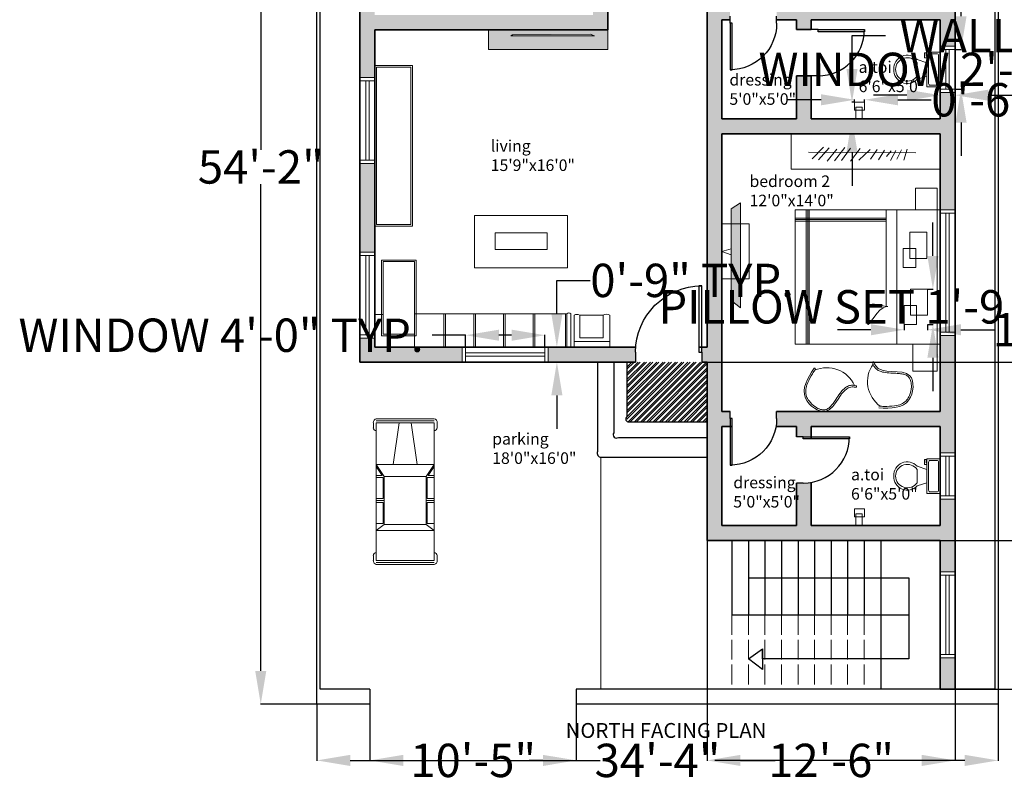
# Model space of a CAD drawing. Units: inches. Extents: x 1202 to 2101, y 998 to 1743.
# Tile 1 of 4: x 1202 to 1798, y 998 to 1460. Entities that reach past the tile are written whole.
import ezdxf

# ---------------------------------------------------------------- set-up
doc = ezdxf.new("R2010")
doc.units = ezdxf.units.IN
doc.header["$MEASUREMENT"] = 0
doc.linetypes.add('ACAD_ISO02W100', pattern=[15, 12, -3])
for name, color, linetype, lineweight in [('A-ANNO-DIMS', 2, 'Continuous', 18), ('A-ANNO-TEXT', 7, 'Continuous', 18), ('A-AREA-IDEN', 7, 'Continuous', 18), ('A-DOOR', 3, 'Continuous', 25), ('A-FLOR-CASE', 8, 'Continuous', 18), ('A-FLOR-FIXT', 9, 'Continuous', 18), ('A-FLOR-PATT', 9, 'Continuous', 13), ('A-FLOR-STRS', 7, 'Continuous', 25), ('A-FLOR-STRS-OVHD', 8, 'ACAD_ISO02W100', 18), ('A-FURN', 8, 'Continuous', 18), ('A-FURN-PATT', 250, 'Continuous', 13), ('A-GLAZ', 4, 'Continuous', 18), ('A-SITE-VEHC', 8, 'Continuous', 13), ('A-WALL', 7, 'Continuous', 35), ('A-WALL-PATT', 250, 'Continuous', 13), ('C-PROP', 7, 'Continuous', 30), ('C-PVMT', 8, 'Continuous', 18)]:
    doc.layers.add(name, color=color, linetype=linetype, lineweight=lineweight)
doc.styles.get("Standard").update_dxf_attribs({"font": 'arial.ttf'})
doc.dimstyles.get("Standard").update_dxf_attribs({"dimtxt": 20.18, "dimasz": 20.18, "dimexe": 0.18, "dimexo": 0.0625, "dimgap": 0.09, "dimtad": 0, "dimtih": 1, "dimtoh": 1, "dimdec": 0, "dimzin": 0, "dimdsep": 46, "dimlunit": 3, "dimtxsty": 'Standard', "dimcen": 0.09, "dimadec": 0, "dimazin": 0, "dimtfac": 1, "dimtdec": 0, "dimtofl": 0, "dimtmove": 0, "dimatfit": 3, "dimfxl": 1, "dimtolj": 1, "dimtzin": 0, "dimarcsym": 0})

# ---------------------------------------------------------------- blocks, each defined once
blk = doc.blocks.new('*U2')
for p, q in [((0, 0), (0, -6)), ((40, 0), (40, -6))]:
    blk.add_line(p, q)
blk.add_lwpolyline([(0, 0), (0, 40), (1.75, 40), (1.75, 0)], close=True)
blk.add_arc((0, 0), 40, 0, 90)
blk = doc.blocks.new('*U11')
for p, q in [((5.4, 42.3), (12.1, 42.3)), ((189.7, 42.3), (183, 42.3)), ((0.1, -0.4), (0.1, 38.3)), ((2.8, -0.4), (2.8, 38.3)), ((5.4, 38.3), (16.1, 38.3)), ((5.4, -0.4), (5.4, 38.2)), ((16.1, 38.3), (180.3, 38.3)), ((61.5, -0.4), (61.5, 38.3)), ((61.5, 38.3), (77.5, 27.6)), ((64.2, 38.3), (76.2, 30.3)), ((76.2, 30.3), (76.2, 38.3)), ((77.5, 27.6), (141.6, 27.6)), ((77.5, -0.4), (77.5, 27.6)), ((78.9, 38.3), (78.9, 29)), ((78.9, 29), (106.9, 29)), ((106.9, 29), (106.9, 38.3)), ((109.6, 27.6), (109.6, 38.3)), ((112.3, 38.3), (112.3, 29)), ((112.3, 29), (140.3, 29)), ((140.3, 29), (140.3, 38.3)), ((141.6, 27.6), (149.6, 38.3)), ((141.6, -0.4), (141.6, 27.6)), ((149.6, -0.4), (149.6, 38.3)), ((189.7, 38.3), (179, 38.3)), ((189.7, -0.4), (189.7, 38.2)), ((192.4, -0.4), (192.4, 38.3)), ((195, -0.4), (195, 38.3)), ((5.4, 7.6), (61.5, 15.6)), ((0.1, -0.4), (0.1, -39.2)), ((2.8, -0.4), (2.8, -39.1)), ((5.4, -0.4), (5.4, -39.1)), ((5.4, -8.4), (61.5, -16.4)), ((61.5, -0.4), (61.5, -39.1)), ((77.5, -0.4), (77.5, -28.5)), ((141.6, -0.4), (141.6, -28.5)), ((149.6, -0.4), (149.6, -39.1)), ((189.7, -0.4), (189.7, -39.1)), ((192.4, -0.4), (192.4, -39.1)), ((195, -0.4), (195, -39.2)), ((5.4, -39.1), (16.1, -39.1)), ((16.1, -39.1), (180.3, -39.1)), ((61.5, -39.1), (77.5, -28.5)), ((64.2, -39.1), (76.2, -31.1)), ((76.2, -31.1), (76.2, -39.1)), ((77.5, -28.5), (141.6, -28.5)), ((78.9, -39.1), (78.9, -29.8)), ((78.9, -29.8), (106.9, -29.8)), ((106.9, -29.8), (106.9, -39.1)), ((109.6, -28.5), (109.6, -39.1)), ((112.3, -29.8), (140.3, -29.8)), ((112.3, -39.1), (112.3, -29.8)), ((140.3, -29.8), (140.3, -39.1)), ((141.6, -28.5), (149.6, -39.1)), ((189.7, -39.1), (179, -39.1)), ((5.4, -43.1), (12.1, -43.1)), ((189.7, -43.1), (183, -43.1))]:
    blk.add_line(p, q)
for centre, radius, start, end in [((5.1, 37.3), 5.06, 85.6455, 168.0943), ((11.5, 37.6), 4.72, 8.1301, 81.87), ((183.7, 37.6), 4.72, 98.13, 171.8699), ((190.1, 37.3), 5.06, 11.9057, 94.3545), ((5.1, -38.1), 5.06, 191.9057, 274.3545), ((11.5, -38.5), 4.72, 278.13, 351.8699), ((183.7, -38.5), 4.72, 188.1301, 261.87), ((190.1, -38.1), 5.06, 265.6455, 348.0943)]:
    blk.add_arc(centre, radius, start, end)
blk = doc.blocks.new('*U13')
for p, q in [((9.5, -6), (9.5, -2)), ((-10, -8.5), (-8, -8.5)), ((-10, -9.5), (-10, -8.5)), ((-7, -9.5), (-10, -9.5)), ((-8, -8.5), (-8, -8)), ((-7, -8), (-7, -9.5)), ((-4, -8), (-6, -14)), ((4, -8), (6, -14)), ((4, -14), (-4, -14))]:
    blk.add_line(p, q)
blk.add_lwpolyline([(10.5, -8), (10.5, 0), (-10.5, 0), (-10.5, -8)], close=True)
for points in [[(-9.5, -2), (-9.5, -6)], [(8.5, -1), (-8.5, -1)], [(-8.5, -7), (8.5, -7)]]:
    blk.add_lwpolyline(points)
for centre, radius, start, end in [((-8.625, -1.875), 0.8839, 81.8699, 188.1301), ((8.625, -1.875), 0.8839, 351.8699, 98.1301), ((-8.625, -6.125), 0.8839, 171.869898, 278.1301), ((8.625, -6.125), 0.8839, 261.8699, 8.1301), ((-0.4772, -19.9188), 8.0953, 133.01722, 273.38), ((0.0374, -19.8731), 7.127, 124.50543, 269.7), ((-0.0373, -19.8731), 7.127, 270.3, 55.4946), ((0.4773, -19.9188), 8.0953, 266.62, 46.9828)]:
    blk.add_arc(centre, radius, start, end)
blk = doc.blocks.new('WIN-48IN-PLAN')
for p, q in [((9, 48), (0, 48)), ((3.5, 48), (3.5, 0)), ((5.5, 48), (5.5, 0)), ((9, 0), (0, 0))]:
    blk.add_line(p, q)
blk = doc.blocks.new('WIN-24IN-PLAN')
for p, q in [((0, 24), (9, 24)), ((3.5, 24), (3.5, 0)), ((5.5, 24), (5.5, 0)), ((0, 0), (9, 0))]:
    blk.add_line(p, q)
blk = doc.blocks.new('BATH-WALL-FITTING')
for p, q in [((0.87, 0), (0.87, 7.15)), ((0.87, 7.15), (4.62, 7.15)), ((4.62, 7.15), (4.62, 0))]:
    blk.add_line(p, q)
blk.add_lwpolyline([(0, 10.11), (6.07, 10.11), (6.07, 5.36), (0, 5.36)], close=True)
blk = doc.blocks.new('BED-PILLOW-SET')
for points in [[(3.88, 21.33), (14.16, 21.33), (14.16, 5.54), (3.88, 5.54)], [(7.51, 11.51), (0, 11.51), (0, 0), (7.51, 0)]]:
    blk.add_lwpolyline(points, close=True)
blk = doc.blocks.new('*D19')
at = {"layer": 'A-ANNO-DIMS', "color": 0, "lineweight": -2, "transparency": 16777216}
for p, q in [((1471.91, 1268.67), (1451.73, 1268.67)), ((1471.91, 1261.53), (1471.91, 1268.85)), ((1499.73, 1268.67), (1492.09, 1268.67)), ((1519.91, 1261.53), (1519.91, 1268.85))]:
    blk.add_line(p, q, dxfattribs=at)
at = {"layer": 'A-ANNO-DIMS', "color": 0, "transparency": 16777216}
for points in [[(1492.09, 1272.03), (1492.09, 1265.3), (1471.91, 1268.67)], [(1499.73, 1272.03), (1499.73, 1265.3), (1519.91, 1268.67)]]:
    blk.add_solid(points, dxfattribs=at)
at = {"layer": 'Defpoints', "color": 0, "transparency": 16777216}
for p in [(1471.91, 1268.67), (1471.91, 1261.47), (1519.91, 1261.47)]:
    blk.add_point(p, dxfattribs=at)
at = {"layer": 'A-ANNO-DIMS', "color": 0, "transparency": 16777216, "insert": (1323.96, 1268.67), "char_height": 20.18, "attachment_point": 5}
blk.add_mtext('\\A1;WINDOW 4\'-0" TYP.', dxfattribs=at)
blk = doc.blocks.new('*D20')
at = {"layer": 'A-ANNO-DIMS', "color": 0, "lineweight": -2, "transparency": 16777216}
for p, q in [((1527.11, 1281.65), (1527.11, 1301.83)), ((1527.11, 1301.83), (1547.29, 1301.83)), ((1519.98, 1261.47), (1527.29, 1261.47)), ((1519.98, 1252.47), (1527.29, 1252.47)), ((1527.11, 1232.29), (1527.11, 1212.11))]:
    blk.add_line(p, q, dxfattribs=at)
at = {"layer": 'A-ANNO-DIMS', "color": 0, "transparency": 16777216}
for points in [[(1523.75, 1281.65), (1530.48, 1281.65), (1527.11, 1261.47)], [(1523.75, 1232.29), (1530.48, 1232.29), (1527.11, 1252.47)]]:
    blk.add_solid(points, dxfattribs=at)
at = {"layer": 'Defpoints', "color": 0, "transparency": 16777216}
for p in [(1519.91, 1261.47), (1527.11, 1261.47), (1519.91, 1252.47)]:
    blk.add_point(p, dxfattribs=at)
at = {"layer": 'A-ANNO-DIMS', "color": 0, "transparency": 16777216, "insert": (1608.89, 1301.83), "char_height": 20.18, "attachment_point": 5}
blk.add_mtext('\\A1;0\'-9" TYP.', dxfattribs=at)
blk = doc.blocks.new('*D21')
at = {"layer": 'A-ANNO-DIMS', "color": 0, "lineweight": -2, "transparency": 16777216}
for p, q in [((1771.58, 1461.65), (1771.58, 1481.83)), ((1768.04, 1441.47), (1771.76, 1441.47)), ((1768.04, 1417.47), (1771.76, 1417.47)), ((1771.58, 1397.29), (1771.58, 1377.11))]:
    blk.add_line(p, q, dxfattribs=at)
at = {"layer": 'A-ANNO-DIMS', "color": 0, "transparency": 16777216}
for points in [[(1768.21, 1461.65), (1774.94, 1461.65), (1771.58, 1441.47)], [(1768.21, 1397.29), (1774.94, 1397.29), (1771.58, 1417.47)]]:
    blk.add_solid(points, dxfattribs=at)
at = {"layer": 'Defpoints', "color": 0, "transparency": 16777216}
for p in [(1767.98, 1441.47), (1771.58, 1441.47), (1767.98, 1417.47)]:
    blk.add_point(p, dxfattribs=at)
at = {"layer": 'A-ANNO-DIMS', "color": 0, "transparency": 16777216, "insert": (1771.58, 1429.47), "char_height": 20.18, "attachment_point": 5}
blk.add_mtext('\\A1;WINDOW 2\'-0" TYP.', dxfattribs=at)
blk = doc.blocks.new('*D22')
at = {"layer": 'A-ANNO-DIMS', "color": 0, "lineweight": -2, "transparency": 16777216}
for p, q in [((1738.8, 1413.87), (1718.62, 1413.87)), ((1758.98, 1417.4), (1758.98, 1413.69)), ((1767.98, 1417.4), (1767.98, 1413.69)), ((1788.16, 1413.87), (1808.34, 1413.87))]:
    blk.add_line(p, q, dxfattribs=at)
at = {"layer": 'A-ANNO-DIMS', "color": 0, "transparency": 16777216}
for points in [[(1738.8, 1417.23), (1738.8, 1410.5), (1758.98, 1413.87)], [(1788.16, 1417.23), (1788.16, 1410.5), (1767.98, 1413.87)]]:
    blk.add_solid(points, dxfattribs=at)
at = {"layer": 'Defpoints', "color": 0, "transparency": 16777216}
for p in [(1758.98, 1417.47), (1767.98, 1417.47), (1767.98, 1413.87)]:
    blk.add_point(p, dxfattribs=at)
at = {"layer": 'A-ANNO-DIMS', "color": 0, "transparency": 16777216, "insert": (1869.93, 1413.87), "char_height": 20.18, "attachment_point": 5}
blk.add_mtext('\\A1;0\'-9" TYP.', dxfattribs=at)
blk = doc.blocks.new('*D23')
at = {"layer": 'A-ANNO-DIMS', "color": 0, "lineweight": -2, "transparency": 16777216}
for p, q in [((1705.63, 1429.75), (1705.63, 1449.93)), ((1705.63, 1449.93), (1725.81, 1449.93)), ((1707.09, 1409.57), (1705.45, 1409.57)), ((1707.09, 1399.47), (1705.45, 1399.47)), ((1705.63, 1379.29), (1705.63, 1359.11))]:
    blk.add_line(p, q, dxfattribs=at)
at = {"layer": 'A-ANNO-DIMS', "color": 0, "transparency": 16777216}
for points in [[(1702.27, 1429.75), (1709, 1429.75), (1705.63, 1409.57)], [(1702.27, 1379.29), (1709, 1379.29), (1705.63, 1399.47)]]:
    blk.add_solid(points, dxfattribs=at)
at = {"layer": 'Defpoints', "color": 0, "transparency": 16777216}
for p in [(1705.63, 1409.57), (1707.15, 1409.57), (1707.15, 1399.47)]:
    blk.add_point(p, dxfattribs=at)
at = {"layer": 'A-ANNO-DIMS', "color": 0, "transparency": 16777216, "insert": (1896.68, 1449.93), "char_height": 20.18, "attachment_point": 5}
blk.add_mtext('\\A1;WALL FITTING 0\'-10" TYP.', dxfattribs=at)
blk = doc.blocks.new('*D24')
at = {"layer": 'A-ANNO-DIMS', "color": 0, "lineweight": -2, "transparency": 16777216}
for p, q in [((1686.97, 1411.09), (1666.79, 1411.09)), ((1707.15, 1409.64), (1707.15, 1411.27)), ((1713.22, 1409.64), (1713.22, 1411.27)), ((1733.4, 1411.09), (1753.58, 1411.09))]:
    blk.add_line(p, q, dxfattribs=at)
at = {"layer": 'A-ANNO-DIMS', "color": 0, "transparency": 16777216}
for points in [[(1686.97, 1414.45), (1686.97, 1407.73), (1707.15, 1411.09)], [(1733.4, 1414.45), (1733.4, 1407.73), (1713.22, 1411.09)]]:
    blk.add_solid(points, dxfattribs=at)
at = {"layer": 'Defpoints', "color": 0, "transparency": 16777216}
for p in [(1707.15, 1409.57), (1713.22, 1411.09), (1713.22, 1409.57)]:
    blk.add_point(p, dxfattribs=at)
at = {"layer": 'A-ANNO-DIMS', "color": 0, "transparency": 16777216, "insert": (1815.17, 1411.09), "char_height": 20.18, "attachment_point": 5}
blk.add_mtext('\\A1;0\'-6" TYP.', dxfattribs=at)
blk = doc.blocks.new('*D25')
at = {"layer": 'A-ANNO-DIMS', "color": 0, "lineweight": -2, "transparency": 16777216}
for p, q in [((1754.58, 1316.69), (1754.58, 1336.87)), ((1751.44, 1296.51), (1754.76, 1296.51)), ((1751.44, 1275.18), (1754.76, 1275.18)), ((1754.58, 1255), (1754.58, 1234.82))]:
    blk.add_line(p, q, dxfattribs=at)
at = {"layer": 'A-ANNO-DIMS', "color": 0, "transparency": 16777216}
for points in [[(1751.22, 1316.69), (1757.94, 1316.69), (1754.58, 1296.51)], [(1751.22, 1255), (1757.94, 1255), (1754.58, 1275.18)]]:
    blk.add_solid(points, dxfattribs=at)
at = {"layer": 'Defpoints', "color": 0, "transparency": 16777216}
for p in [(1751.38, 1296.51), (1754.58, 1296.51), (1751.38, 1275.18)]:
    blk.add_point(p, dxfattribs=at)
at = {"layer": 'A-ANNO-DIMS', "color": 0, "transparency": 16777216, "insert": (1754.58, 1285.85), "char_height": 20.18, "attachment_point": 5}
blk.add_mtext('\\A1;PILLOW SET 1\'-9 1/2" TYP.', dxfattribs=at)
blk = doc.blocks.new('*D26')
at = {"layer": 'A-ANNO-DIMS', "color": 0, "lineweight": -2, "transparency": 16777216}
for p, q in [((1737.22, 1275.12), (1737.22, 1271.8)), ((1751.38, 1275.12), (1751.38, 1271.8)), ((1717.04, 1271.98), (1696.86, 1271.98)), ((1771.56, 1271.98), (1791.74, 1271.98))]:
    blk.add_line(p, q, dxfattribs=at)
at = {"layer": 'A-ANNO-DIMS', "color": 0, "transparency": 16777216}
for points in [[(1717.04, 1275.35), (1717.04, 1268.62), (1737.22, 1271.98)], [(1771.56, 1275.35), (1771.56, 1268.62), (1751.38, 1271.98)]]:
    blk.add_solid(points, dxfattribs=at)
at = {"layer": 'Defpoints', "color": 0, "transparency": 16777216}
for p in [(1737.22, 1275.18), (1751.38, 1275.18), (1751.38, 1271.98)]:
    blk.add_point(p, dxfattribs=at)
at = {"layer": 'A-ANNO-DIMS', "color": 0, "transparency": 16777216, "insert": (1852.38, 1271.98), "char_height": 20.18, "attachment_point": 5}
blk.add_mtext('\\A1;1\'-2" TYP.', dxfattribs=at)
blk = doc.blocks.new('*D27')
at = {"layer": 'A-ANNO-DIMS', "color": 0, "lineweight": -2, "transparency": 16777216}
for p, q in [((1719.4, 1502.04), (1699.22, 1502.04)), ((1739.58, 1504.38), (1739.58, 1501.86)), ((1755.58, 1504.38), (1755.58, 1501.86)), ((1775.76, 1502.04), (1795.94, 1502.04))]:
    blk.add_line(p, q, dxfattribs=at)
at = {"layer": 'A-ANNO-DIMS', "color": 0, "transparency": 16777216}
for points in [[(1719.4, 1505.41), (1719.4, 1498.68), (1739.58, 1502.04)], [(1775.76, 1505.41), (1775.76, 1498.68), (1755.58, 1502.04)]]:
    blk.add_solid(points, dxfattribs=at)
at = {"layer": 'Defpoints', "color": 0, "transparency": 16777216}
for p in [(1739.58, 1504.44), (1755.58, 1504.44), (1755.58, 1502.04)]:
    blk.add_point(p, dxfattribs=at)
at = {"layer": 'A-ANNO-DIMS', "color": 0, "transparency": 16777216, "insert": (1952.58, 1502.04), "char_height": 20.18, "attachment_point": 5}
blk.add_mtext('\\A1;NIGHTSTAND 1\'-4" TYP.', dxfattribs=at)
blk = doc.blocks.new('*D39')
at = {"layer": 'A-ANNO-DIMS', "color": 0, "lineweight": -2, "transparency": 16777216}
for p, q in [((1381.98, 1045.4), (1381.98, 1011.29)), ((1793.98, 1045.4), (1793.98, 1011.29)), ((1402.16, 1011.47), (1553.23, 1011.47)), ((1773.8, 1011.47), (1622.72, 1011.47))]:
    blk.add_line(p, q, dxfattribs=at)
at = {"layer": 'A-ANNO-DIMS', "color": 0, "transparency": 16777216}
for points in [[(1402.16, 1014.83), (1402.16, 1008.1), (1381.98, 1011.47)], [(1773.8, 1014.83), (1773.8, 1008.1), (1793.98, 1011.47)]]:
    blk.add_solid(points, dxfattribs=at)
at = {"layer": 'Defpoints', "color": 0, "transparency": 16777216}
for p in [(1381.98, 1045.47), (1793.98, 1045.47), (1793.98, 1011.47)]:
    blk.add_point(p, dxfattribs=at)
at = {"layer": 'A-ANNO-DIMS', "color": 0, "transparency": 16777216, "insert": (1587.98, 1011.47), "char_height": 20.18, "attachment_point": 5}
blk.add_mtext('\\A1;34\'-4"', dxfattribs=at)
blk = doc.blocks.new('*D40')
at = {"layer": 'A-ANNO-DIMS', "color": 0, "lineweight": -2, "transparency": 16777216}
for p, q in [((1381.91, 1695.47), (1347.8, 1695.47)), ((1347.98, 1675.29), (1347.98, 1380.86)), ((1347.98, 1065.65), (1347.98, 1360.07)), ((1381.91, 1045.47), (1347.8, 1045.47))]:
    blk.add_line(p, q, dxfattribs=at)
at = {"layer": 'A-ANNO-DIMS', "color": 0, "transparency": 16777216}
for points in [[(1344.61, 1675.29), (1351.34, 1675.29), (1347.98, 1695.47)], [(1344.61, 1065.65), (1351.34, 1065.65), (1347.98, 1045.47)]]:
    blk.add_solid(points, dxfattribs=at)
at = {"layer": 'Defpoints', "color": 0, "transparency": 16777216}
for p in [(1347.98, 1695.47), (1381.98, 1695.47), (1381.98, 1045.47)]:
    blk.add_point(p, dxfattribs=at)
at = {"layer": 'A-ANNO-DIMS', "color": 0, "transparency": 16777216, "insert": (1347.98, 1370.47), "char_height": 20.18, "attachment_point": 5}
blk.add_mtext('\\A1;54\'-2"', dxfattribs=at)
blk = doc.blocks.new('*D41')
at = {"layer": 'A-ANNO-DIMS', "color": 0, "lineweight": -2, "transparency": 16777216}
for p, q in [((1618.04, 1252.47), (1853.16, 1252.47)), ((1852.98, 1232.29), (1852.98, 1208.86)), ((1852.98, 1164.65), (1852.98, 1188.07)), ((1759.04, 1144.47), (1853.16, 1144.47))]:
    blk.add_line(p, q, dxfattribs=at)
at = {"layer": 'A-ANNO-DIMS', "color": 0, "transparency": 16777216}
for points in [[(1849.61, 1232.29), (1856.34, 1232.29), (1852.98, 1252.47)], [(1849.61, 1164.65), (1856.34, 1164.65), (1852.98, 1144.47)]]:
    blk.add_solid(points, dxfattribs=at)
at = {"layer": 'Defpoints', "color": 0, "transparency": 16777216}
for p in [(1617.98, 1252.47), (1852.98, 1252.47), (1758.98, 1144.47)]:
    blk.add_point(p, dxfattribs=at)
at = {"layer": 'A-ANNO-DIMS', "color": 0, "transparency": 16777216, "insert": (1852.98, 1198.47), "char_height": 20.18, "attachment_point": 5}
blk.add_mtext('\\A1;9\'-0"', dxfattribs=at)
blk = doc.blocks.new('*D42')
at = {"layer": 'A-ANNO-DIMS', "color": 0, "lineweight": -2, "transparency": 16777216}
for p, q in [((1768.04, 1669.47), (1853.16, 1669.47)), ((1852.98, 1649.29), (1852.98, 1471.37)), ((1852.98, 1272.65), (1852.98, 1450.57)), ((1618.04, 1252.47), (1853.16, 1252.47))]:
    blk.add_line(p, q, dxfattribs=at)
at = {"layer": 'A-ANNO-DIMS', "color": 0, "transparency": 16777216}
for points in [[(1849.61, 1649.29), (1856.34, 1649.29), (1852.98, 1669.47)], [(1849.61, 1272.65), (1856.34, 1272.65), (1852.98, 1252.47)]]:
    blk.add_solid(points, dxfattribs=at)
at = {"layer": 'Defpoints', "color": 0, "transparency": 16777216}
for p in [(1767.98, 1669.47), (1852.98, 1669.47), (1617.98, 1252.47)]:
    blk.add_point(p, dxfattribs=at)
at = {"layer": 'A-ANNO-DIMS', "color": 0, "transparency": 16777216, "insert": (1852.98, 1460.97), "char_height": 20.18, "attachment_point": 5}
blk.add_mtext('\\A1;34\'-9"', dxfattribs=at)
blk = doc.blocks.new('*D44')
at = {"layer": 'A-ANNO-DIMS', "color": 0, "lineweight": -2, "transparency": 16777216}
for p, q in [((1414.05, 1045.4), (1414.05, 1011.29)), ((1538.87, 1045.4), (1538.87, 1011.29)), ((1434.23, 1011.47), (1442.66, 1011.47)), ((1518.69, 1011.47), (1510.26, 1011.47))]:
    blk.add_line(p, q, dxfattribs=at)
at = {"layer": 'A-ANNO-DIMS', "color": 0, "transparency": 16777216}
for points in [[(1434.23, 1014.83), (1434.23, 1008.1), (1414.05, 1011.47)], [(1518.69, 1014.83), (1518.69, 1008.1), (1538.87, 1011.47)]]:
    blk.add_solid(points, dxfattribs=at)
at = {"layer": 'Defpoints', "color": 0, "transparency": 16777216}
for p in [(1414.05, 1045.47), (1538.87, 1045.47), (1538.87, 1011.47)]:
    blk.add_point(p, dxfattribs=at)
at = {"layer": 'A-ANNO-DIMS', "color": 0, "transparency": 16777216, "insert": (1476.46, 1011.47), "char_height": 20.18, "attachment_point": 5}
blk.add_mtext('\\A1;10\'-5"', dxfattribs=at)
blk = doc.blocks.new('*D46')
at = {"layer": 'A-ANNO-DIMS', "color": 0, "lineweight": -2, "transparency": 16777216}
for p, q in [((1759.04, 1144.47), (1853.16, 1144.47)), ((1852.98, 1124.29), (1852.98, 1109.86)), ((1852.98, 1074.65), (1852.98, 1089.07)), ((1759.04, 1054.47), (1853.16, 1054.47))]:
    blk.add_line(p, q, dxfattribs=at)
at = {"layer": 'A-ANNO-DIMS', "color": 0, "transparency": 16777216}
for points in [[(1849.61, 1124.29), (1856.34, 1124.29), (1852.98, 1144.47)], [(1849.61, 1074.65), (1856.34, 1074.65), (1852.98, 1054.47)]]:
    blk.add_solid(points, dxfattribs=at)
at = {"layer": 'Defpoints', "color": 0, "transparency": 16777216}
for p in [(1758.98, 1144.47), (1852.98, 1144.47), (1758.98, 1054.47)]:
    blk.add_point(p, dxfattribs=at)
at = {"layer": 'A-ANNO-DIMS', "color": 0, "transparency": 16777216, "insert": (1852.98, 1099.47), "char_height": 20.18, "attachment_point": 5}
blk.add_mtext('\\A1;7\'-6"', dxfattribs=at)
blk = doc.blocks.new('*D47')
at = {"layer": 'A-ANNO-DIMS', "color": 0, "lineweight": -2, "transparency": 16777216}
for p, q in [((1617.98, 1144.4), (1617.98, 1011.29)), ((1767.98, 1054.4), (1767.98, 1011.29)), ((1638.16, 1011.47), (1659.18, 1011.47)), ((1747.8, 1011.47), (1726.78, 1011.47))]:
    blk.add_line(p, q, dxfattribs=at)
at = {"layer": 'A-ANNO-DIMS', "color": 0, "transparency": 16777216}
for points in [[(1638.16, 1014.83), (1638.16, 1008.1), (1617.98, 1011.47)], [(1747.8, 1014.83), (1747.8, 1008.1), (1767.98, 1011.47)]]:
    blk.add_solid(points, dxfattribs=at)
at = {"layer": 'Defpoints', "color": 0, "transparency": 16777216}
for p in [(1617.98, 1144.47), (1767.98, 1054.47), (1767.98, 1011.47)]:
    blk.add_point(p, dxfattribs=at)
at = {"layer": 'A-ANNO-DIMS', "color": 0, "transparency": 16777216, "insert": (1692.98, 1011.47), "char_height": 20.18, "attachment_point": 5}
blk.add_mtext('\\A1;12\'-6"', dxfattribs=at)

msp = doc.modelspace()

# ---------------------------------------------------------------- hatches: boundary and pattern name
at = {"layer": 'A-FLOR-PATT'}
h = msp.add_hatch(dxfattribs=at)
h.set_pattern_fill('ANSI32', color=256, scale=7.1)
h.paths.add_polyline_path([(1617.98, 1252.47), (1614.74, 1252.47), (1569.41, 1252.47), (1569.41, 1216.34), (1617.98, 1216.34)])
at = {"layer": 'A-FURN-PATT'}
h = msp.add_hatch(color=256, dxfattribs=at)
h.dxf.hatch_style = 1
h.paths.add_polyline_path([(1557.98, 1453.47), (1485.75, 1453.47), (1485.75, 1441.44), (1557.98, 1441.44)])
h.paths.add_polyline_path([(1500.3, 1450.41), (1499.23, 1449.68), (1549.91, 1449.68), (1547.28, 1450.79)], flags=16)
h = msp.add_hatch(color=256, dxfattribs=at)
h.dxf.hatch_style = 1
h.paths.add_polyline_path([(1638.27, 1335.98), (1632.52, 1335.98), (1632.52, 1302.7), (1638.27, 1302.7)])
h.paths.add_polyline_path([(1638.27, 1348.82), (1632.52, 1345.06), (1632.52, 1335.98), (1638.27, 1335.98)])
h.paths.add_polyline_path([(1638.27, 1302.7), (1632.52, 1302.7), (1632.52, 1289.65), (1638.27, 1285.22)])
at = {"layer": 'A-WALL-PATT'}
h = msp.add_hatch(color=256, dxfattribs=at)
h.dxf.hatch_style = 1
h.paths.add_polyline_path([(1767.98, 1669.47), (1407.98, 1669.47), (1407.98, 1552.97), (1416.98, 1552.97), (1416.98, 1591.47), (1527.46, 1591.47), (1527.46, 1600.47), (1416.98, 1600.47), (1416.98, 1660.47), (1548.98, 1660.47), (1548.98, 1600.47), (1544.75, 1600.47), (1544.75, 1591.47), (1548.98, 1591.47), (1548.98, 1584.29), (1557.98, 1584.29), (1557.98, 1660.47), (1617.98, 1660.47), (1617.98, 1540.47), (1557.98, 1540.47), (1557.98, 1544.29), (1548.98, 1544.29), (1548.98, 1462.47), (1416.98, 1462.47), (1416.98, 1500.97), (1407.98, 1500.97), (1407.98, 1424.63), (1416.98, 1424.63), (1416.98, 1431.74), (1416.98, 1453.47), (1557.98, 1453.47), (1557.98, 1531.47), (1617.98, 1531.47), (1617.98, 1507.47), (1622.48, 1507.47, -0.014283), (1624.48, 1507.47), (1626.98, 1507.47), (1626.98, 1660.47), (1758.98, 1660.47), (1758.98, 1638.32), (1758.98, 1561.97), (1767.98, 1561.97)])
h.paths.add_polyline_path([(1416.98, 1372.63), (1407.98, 1372.63), (1407.98, 1318.84), (1416.98, 1318.84)])
h.paths.add_polyline_path([(1626.98, 1390.47), (1758.98, 1390.47), (1758.98, 1369.1), (1758.98, 1344.47), (1767.98, 1344.47), (1767.98, 1415.47), (1758.98, 1415.47), (1758.98, 1399.47), (1680.98, 1399.47), (1680.98, 1425.58), (1671.98, 1425.58), (1671.98, 1399.47), (1626.98, 1399.47), (1626.98, 1459.47), (1631.88, 1459.47), (1631.88, 1461.58), (1631.88, 1468.47), (1626.98, 1468.47), (1626.98, 1471.47), (1622.48, 1471.47), (1617.98, 1471.47), (1617.98, 1261.47), (1614.74, 1261.47), (1614.74, 1258.47), (1614.74, 1252.47), (1617.98, 1252.47), (1617.98, 1144.47), (1758.98, 1144.47), (1758.98, 1125.47), (1767.98, 1125.47), (1767.98, 1169.47), (1758.98, 1169.47), (1758.98, 1153.47), (1680.98, 1153.47), (1680.98, 1179.68, -0.04329), (1676.17, 1179.26), (1671.98, 1179.26), (1671.98, 1153.47), (1626.98, 1153.47), (1626.98, 1213.47), (1631.88, 1213.47), (1631.88, 1218.24), (1631.88, 1222.47), (1626.98, 1222.47)])
h.paths.add_polyline_path([(1767.98, 1509.97), (1758.98, 1509.97), (1758.98, 1468.47), (1660.05, 1468.47), (1660.05, 1461.58), (1660.05, 1459.47), (1671.98, 1459.47), (1671.98, 1453.51), (1680.98, 1453.51), (1680.98, 1459.47), (1758.98, 1459.47), (1758.98, 1443.47), (1767.98, 1443.47)], flags=17)
h.paths.add_polyline_path([(1767.98, 1268.47), (1758.98, 1268.47), (1758.98, 1263.28), (1758.98, 1222.47), (1660.05, 1222.47), (1660.05, 1218.24, -0.04262), (1659.64, 1213.47), (1671.98, 1213.47), (1671.98, 1207.19), (1676.17, 1207.19), (1680.98, 1207.19), (1680.98, 1213.47), (1758.98, 1213.47), (1758.98, 1197.47), (1767.98, 1197.47)], flags=17)
h.paths.add_polyline_path([(1767.98, 1073.47), (1758.98, 1073.47), (1758.98, 1054.47), (1767.98, 1054.47)])
h = msp.add_hatch(color=256, dxfattribs=at)
h.dxf.hatch_style = 1
h.paths.add_polyline_path([(1469.91, 1261.47), (1440.99, 1261.47), (1416.98, 1261.47), (1416.98, 1266.84), (1407.98, 1266.84), (1407.98, 1252.47), (1469.91, 1252.47)])
h.paths.add_polyline_path([(1574.74, 1258.47, -0.01877), (1574.85, 1261.47), (1521.91, 1261.47), (1521.91, 1252.47), (1574.74, 1252.47)])

# ---------------------------------------------------------------- linework, layer by layer
at = {"layer": 'A-FLOR-CASE'}
for p, q in [((1681.49, 1375.36), (1688.4, 1382.38)), ((1685.44, 1374.86), (1691.73, 1382.01)), ((1695.06, 1374.25), (1701.23, 1382.13)), ((1679.31, 1379.5), (1744.3, 1379.01)), ((1690.62, 1374), (1696.42, 1381.27)), ((1699.26, 1374.37), (1704.68, 1381.76)), ((1704.81, 1373.88), (1710.48, 1381.52)), ((1716.53, 1381.02), (1709.74, 1374.62)), ((1720.85, 1380.92), (1716.81, 1375.19)), ((1725.19, 1380.69), (1721.7, 1374.72)), ((1729.38, 1380.3), (1726.51, 1376.74)), ((1732.1, 1380.46), (1728.84, 1374.34)), ((1735.51, 1380.77), (1732.8, 1375.19)), ((1739, 1381.23), (1737.06, 1374.65))]:
    msp.add_line(p, q, dxfattribs=at)
msp.add_lwpolyline([(1758.98, 1390.47), (1668.9, 1390.47), (1668.9, 1369.1), (1758.98, 1369.1)], close=True, dxfattribs=at)
at = {"layer": 'A-FLOR-STRS'}
for p, q in [((1551.73, 1252.47), (1551.73, 1198.3)), ((1561.52, 1252.47), (1561.52, 1209.7)), ((1569.41, 1252.47), (1569.41, 1219.23)), ((1570.28, 1216.34), (1617.98, 1216.34)), ((1564.31, 1206.88), (1617.98, 1206.88)), ((1553.69, 1194.9), (1617.98, 1194.9)), ((1632.98, 1144.47), (1632.98, 1099.47)), ((1642.98, 1144.47), (1642.98, 1099.47)), ((1652.98, 1144.47), (1652.98, 1099.47)), ((1652.98, 1144.47), (1652.98, 1099.47)), ((1662.98, 1144.47), (1662.98, 1099.47)), ((1662.98, 1144.47), (1662.98, 1099.47)), ((1672.98, 1144.47), (1672.98, 1099.47)), ((1672.98, 1144.47), (1672.98, 1099.47)), ((1682.98, 1144.47), (1682.98, 1099.47)), ((1682.98, 1144.47), (1682.98, 1099.47)), ((1682.98, 1144.47), (1682.98, 1099.47)), ((1682.98, 1144.47), (1682.98, 1099.47)), ((1682.98, 1144.47), (1682.98, 1099.47)), ((1692.98, 1144.47), (1692.98, 1099.47)), ((1692.98, 1144.47), (1692.98, 1099.47)), ((1702.98, 1144.47), (1702.98, 1099.47)), ((1702.98, 1144.47), (1702.98, 1099.47)), ((1712.98, 1144.47), (1712.98, 1099.47)), ((1712.98, 1144.47), (1712.98, 1099.47)), ((1722.98, 1144.47), (1722.98, 1054.47)), ((1642.98, 1121.97), (1740, 1121.97)), ((1740, 1121.97), (1740, 1072.83)), ((1632.98, 1099.47), (1740, 1099.47)), ((1642.98, 1072.98), (1651.4, 1078.9)), ((1651.4, 1072.83), (1651.4, 1078.9)), ((1651.4, 1078.9), (1651.4, 1066.47)), ((1651.4, 1066.47), (1642.98, 1072.98)), ((1740, 1072.83), (1651.4, 1072.83))]:
    msp.add_line(p, q, dxfattribs=at)
for centre, radius, start, end in [((1570.43, 1217.96), 1.63, 128.74153, 275.16789), ((1563.11, 1208.48), 2, 142.57314, 306.98171), ((1553.84, 1197.25), 2.36, 153.49176, 273.58117)]:
    msp.add_arc(centre, radius, start, end, dxfattribs=at)
at = {"layer": 'A-FLOR-STRS-OVHD'}
for p, q in [((1632.98, 1099.47), (1632.98, 1054.47)), ((1642.98, 1099.47), (1642.98, 1054.47)), ((1652.98, 1099.47), (1652.98, 1054.47)), ((1662.98, 1099.47), (1662.98, 1054.47)), ((1672.98, 1099.47), (1672.98, 1054.47)), ((1682.98, 1099.47), (1682.98, 1054.47)), ((1692.98, 1099.47), (1692.98, 1054.47)), ((1702.98, 1099.47), (1702.98, 1054.47)), ((1712.98, 1099.47), (1712.98, 1054.47))]:
    msp.add_line(p, q, dxfattribs=at)
at = {"layer": 'A-FURN'}
for p, q in [((1499.23, 1449.68), (1500.3, 1450.41)), ((1549.91, 1449.68), (1499.23, 1449.68)), ((1500.3, 1450.41), (1547.28, 1450.79)), ((1549.91, 1449.68), (1547.28, 1450.79)), ((1632.52, 1345.06), (1638.27, 1348.82)), ((1638.27, 1348.82), (1638.27, 1285.22)), ((1632.52, 1289.65), (1632.52, 1345.06)), ((1677.81, 1344.47), (1677.81, 1263.28)), ((1678.81, 1344.47), (1678.81, 1263.28)), ((1679.81, 1344.47), (1679.81, 1263.28)), ((1726.38, 1344.47), (1726.38, 1286.01)), ((1732.65, 1344.47), (1732.65, 1263.28)), ((1757.18, 1344.47), (1757.18, 1263.28)), ((1671.2, 1339.57), (1726.38, 1339.57)), ((1671.2, 1338.57), (1726.38, 1338.57)), ((1671.2, 1337.57), (1726.38, 1337.57)), ((1626.98, 1319.34), (1632.52, 1320.83)), ((1626.98, 1319.34), (1632.52, 1317.36)), ((1638.27, 1285.22), (1632.52, 1289.65)), ((1422.02, 1281.2), (1416.98, 1281.2)), ((1458.79, 1281.56), (1458.79, 1261.47)), ((1459.79, 1281.56), (1459.79, 1261.47)), ((1476.79, 1281.56), (1476.79, 1261.47)), ((1477.79, 1281.56), (1477.79, 1261.47)), ((1494.79, 1281.56), (1494.79, 1261.47)), ((1495.79, 1281.56), (1495.79, 1261.47)), ((1512.79, 1281.56), (1512.79, 1261.47)), ((1513.79, 1281.56), (1513.79, 1261.47)), ((1532.33, 1281.56), (1532.33, 1261.47)), ((1532.33, 1281.56), (1533.11, 1281.56)), ((1535.58, 1281.56), (1535.58, 1261.47)), ((1537.54, 1280.76), (1537.54, 1261.47)), ((1559.07, 1280.76), (1559.07, 1261.47)), ((1537.54, 1264.97), (1559.07, 1264.97))]:
    msp.add_line(p, q, dxfattribs=at)
for points in [[(1557.98, 1453.47), (1485.75, 1453.47), (1485.75, 1441.44), (1557.98, 1441.44)], [(1416.98, 1431.74), (1439.81, 1431.74), (1439.81, 1334.63), (1416.98, 1334.63)], [(1417.98, 1430.74), (1438.81, 1430.74), (1438.81, 1335.63), (1417.98, 1335.63)], [(1757.18, 1344.47), (1743.99, 1344.47), (1743.99, 1357.68), (1757.18, 1357.68)], [(1477.22, 1341), (1533.48, 1341), (1533.48, 1309.53), (1477.22, 1309.53)], [(1758.98, 1344.47), (1671.2, 1344.47), (1671.2, 1263.28), (1758.98, 1263.28)], [(1626.98, 1335.98), (1643.44, 1335.98), (1643.44, 1302.7), (1626.98, 1302.7)], [(1489.75, 1330.6), (1521.29, 1330.6), (1521.29, 1320.54), (1489.75, 1320.54)], [(1441.99, 1314.17), (1421.02, 1314.17), (1421.02, 1268.27), (1441.99, 1268.27)], [(1440.99, 1313.17), (1422.02, 1313.17), (1422.02, 1269.27), (1440.99, 1269.27)], [(1440.99, 1281.56), (1533.11, 1281.56), (1533.11, 1261.47), (1440.99, 1261.47)], [(1540.9, 1280.76), (1555.03, 1280.76), (1555.03, 1266.99), (1540.9, 1266.99)], [(1757.18, 1263.28), (1742.46, 1263.28), (1742.46, 1246.83), (1757.18, 1246.83)]]:
    msp.add_lwpolyline(points, close=True, dxfattribs=at)
for centre, radius, start, end in [((1534.35, 1280.65), 1.53, 36.431, 143.569), ((1539.22, 1277.92), 3.3, 59.35125, 120.64875), ((1557.05, 1277.63), 3.72, 57.1692, 122.8308), ((1733.41, 1240.64), 18.38, 145.10534, 234.5049), ((1718.63, 1251.79), 0.776, 68.79867, 149.00785), ((1682.85, 1248.08), 0.665, 8.86727, 106.42873), ((1690.47, 1230.63), 18.38, 24.46294, 113.86249), ((1682.85, 1248.08), 0.665, 286.47397, 300.73646), ((1707.35, 1237.72), 0.98, 317.60073, 18.92097)]:
    msp.add_arc(centre, radius, start, end, dxfattribs=at)
for points, knots in [([(1726.38, 1286.01), (1721.25, 1287.21), (1713.37, 1289.04), (1715.34, 1280.72), (1714.04, 1269.42), (1721.55, 1286.31), (1727.06, 1286.03), (1727.4, 1286.01)], [0, 0, 0, 0, 11.378597, 17.488069, 21.946331, 37.475319, 38.495882, 38.495882, 38.495882, 38.495882]), ([(1721.86, 1225.7), (1722.41, 1225.69), (1722.96, 1225.67), (1724.6, 1225.63), (1725.67, 1225.61), (1728.83, 1225.64), (1730.84, 1225.77), (1733.91, 1226.41), (1735.08, 1226.8), (1737.15, 1227.89), (1738.05, 1228.59), (1739.12, 1229.87), (1739.41, 1230.28), (1739.94, 1231.17), (1740.18, 1231.66), (1741.08, 1233.77), (1741.49, 1235.64), (1741.6, 1238.6), (1741.5, 1239.74), (1741.05, 1241.52), (1740.76, 1242.21), (1740.01, 1243.36), (1739.56, 1243.8), (1738.42, 1244.52), (1737.73, 1244.8), (1736.16, 1245.23), (1735.29, 1245.38), (1733.42, 1245.58), (1732.43, 1245.65), (1729.89, 1245.77), (1728.32, 1245.82), (1725.57, 1246.11), (1724.37, 1246.3), (1722.44, 1246.89), (1721.67, 1247.23), (1720.28, 1248.14), (1719.67, 1248.72), (1719, 1249.71), (1718.85, 1249.99), (1718.57, 1250.55), (1718.45, 1250.84), (1718.21, 1251.49), (1718.09, 1251.84), (1717.97, 1252.19)], [0, 0, 0, 0, 1.423574, 1.423574, 4.270721, 4.270721, 9.965016, 9.965016, 14.007628, 14.007628, 18.050241, 18.050241, 19.670932, 19.670932, 21.291623, 21.291623, 26.38725, 26.38725, 29.733224, 29.733224, 32.363164, 32.363164, 34.993104, 34.993104, 37.623043, 37.623043, 40.252983, 40.252983, 42.882923, 42.882923, 46.855545, 46.855545, 50.084133, 50.084133, 52.435754, 52.435754, 54.787375, 54.787375, 55.637603, 55.637603, 56.487831, 56.487831, 57.549481, 57.549481, 57.549481, 57.549481]), ([(1721.83, 1224.71), (1729.13, 1224.49), (1742.07, 1224.1), (1744.63, 1251.88), (1721.86, 1243.9), (1719.18, 1251.72), (1718.91, 1252.51)], [0, 0, 0, 0, 18.893928, 33.537423, 55.121312, 57.549481, 57.549481, 57.549481, 57.549481]), ([(1682.66, 1248.72), (1678.75, 1242.55), (1671.82, 1231.61), (1694.41, 1215.25), (1699.15, 1238.91), (1707.25, 1237.22), (1708.07, 1237.05)], [0, 0, 0, 0, 18.893928, 33.537423, 55.121312, 57.549481, 57.549481, 57.549481, 57.549481]), ([(1683.5, 1248.18), (1683.21, 1247.72), (1682.92, 1247.25), (1682.05, 1245.87), (1681.48, 1244.95), (1679.89, 1242.22), (1678.98, 1240.42), (1677.97, 1237.45), (1677.71, 1236.25), (1677.59, 1233.92), (1677.73, 1232.79), (1678.29, 1231.21), (1678.5, 1230.75), (1678.99, 1229.84), (1679.29, 1229.39), (1680.65, 1227.54), (1682.05, 1226.23), (1684.54, 1224.62), (1685.57, 1224.13), (1687.33, 1223.61), (1688.08, 1223.51), (1689.44, 1223.57), (1690.05, 1223.73), (1691.25, 1224.35), (1691.85, 1224.79), (1693.02, 1225.92), (1693.59, 1226.6), (1694.72, 1228.11), (1695.27, 1228.93), (1696.68, 1231.04), (1697.52, 1232.37), (1699.17, 1234.59), (1699.94, 1235.53), (1701.44, 1236.88), (1702.12, 1237.37), (1703.61, 1238.1), (1704.43, 1238.34), (1705.61, 1238.41), (1705.93, 1238.4), (1706.56, 1238.34), (1706.87, 1238.3), (1707.55, 1238.19), (1707.92, 1238.11), (1708.27, 1238.03)], [0, 0, 0, 0, 1.423574, 1.423574, 4.270721, 4.270721, 9.965016, 9.965016, 14.007628, 14.007628, 18.050241, 18.050241, 19.670932, 19.670932, 21.291623, 21.291623, 26.38725, 26.38725, 29.733224, 29.733224, 32.363164, 32.363164, 34.993104, 34.993104, 37.623043, 37.623043, 40.252983, 40.252983, 42.882923, 42.882923, 46.855545, 46.855545, 50.084133, 50.084133, 52.435754, 52.435754, 54.787375, 54.787375, 55.637603, 55.637603, 56.487831, 56.487831, 57.549481, 57.549481, 57.549481, 57.549481])]:
    msp.add_open_spline(points, degree=3, knots=knots, dxfattribs=at)
at = {"layer": 'A-GLAZ'}
for p, q in [((1758.98, 1443.47), (1767.98, 1443.47)), ((1416.98, 1424.63), (1407.98, 1424.63)), ((1758.98, 1415.47), (1767.98, 1415.47)), ((1416.98, 1372.63), (1407.98, 1372.63)), ((1758.98, 1344.47), (1767.98, 1344.47)), ((1758.98, 1342.47), (1767.98, 1342.47)), ((1762.48, 1342.47), (1762.48, 1270.47)), ((1764.48, 1342.47), (1764.48, 1270.47)), ((1416.98, 1318.84), (1407.98, 1318.84)), ((1758.98, 1270.47), (1767.98, 1270.47)), ((1416.98, 1266.84), (1407.98, 1266.84)), ((1758.98, 1268.47), (1767.98, 1268.47)), ((1469.91, 1261.47), (1469.91, 1252.47)), ((1521.91, 1261.47), (1521.91, 1252.47)), ((1758.98, 1197.47), (1767.98, 1197.47)), ((1758.98, 1169.47), (1767.98, 1169.47)), ((1758.98, 1125.47), (1767.98, 1125.47)), ((1758.98, 1073.47), (1767.98, 1073.47))]:
    msp.add_line(p, q, dxfattribs=at)
at = {"layer": 'A-WALL'}
for p, q in [((1407.98, 1252.47), (1407.98, 1669.47)), ((1767.98, 1669.47), (1767.98, 1054.47)), ((1557.98, 1453.47), (1557.98, 1531.47)), ((1617.98, 1261.47), (1617.98, 1471.47)), ((1626.98, 1459.47), (1631.88, 1459.47)), ((1626.98, 1399.47), (1626.98, 1459.47)), ((1660.05, 1459.47), (1671.98, 1459.47)), ((1671.98, 1459.47), (1671.98, 1453.51)), ((1680.98, 1459.47), (1680.98, 1453.51)), ((1680.98, 1459.47), (1758.98, 1459.47)), ((1758.98, 1459.47), (1758.98, 1399.47)), ((1416.98, 1453.47), (1557.98, 1453.47)), ((1416.98, 1261.47), (1416.98, 1453.47)), ((1680.98, 1453.51), (1671.98, 1453.51)), ((1680.98, 1425.58), (1671.98, 1425.58)), ((1671.98, 1425.58), (1671.98, 1399.47)), ((1680.98, 1425.58), (1680.98, 1399.47)), ((1626.98, 1399.47), (1671.98, 1399.47)), ((1680.98, 1399.47), (1758.98, 1399.47)), ((1626.98, 1390.47), (1758.98, 1390.47)), ((1626.98, 1222.47), (1626.98, 1390.47)), ((1758.98, 1390.47), (1758.98, 1222.47)), ((1416.98, 1261.47), (1574.85, 1261.47)), ((1612.99, 1261.47), (1617.98, 1261.47)), ((1407.98, 1252.47), (1574.74, 1252.47)), ((1614.74, 1252.47), (1617.98, 1252.47)), ((1617.98, 1144.47), (1617.98, 1252.47)), ((1626.98, 1222.47), (1631.88, 1222.47)), ((1660.05, 1222.47), (1758.98, 1222.47)), ((1626.98, 1213.47), (1633.12, 1213.47)), ((1626.98, 1153.47), (1626.98, 1213.47)), ((1659.64, 1213.47), (1671.98, 1213.47)), ((1671.98, 1213.47), (1671.98, 1207.19)), ((1680.98, 1213.47), (1680.98, 1205.97)), ((1680.98, 1213.47), (1758.98, 1213.47)), ((1758.98, 1213.47), (1758.98, 1153.47)), ((1758.98, 1192.38), (1758.98, 1192.38)), ((1680.98, 1179.68), (1680.98, 1153.47)), ((1671.98, 1179.26), (1671.98, 1153.47)), ((1626.98, 1153.47), (1671.98, 1153.47)), ((1680.98, 1153.47), (1758.98, 1153.47)), ((1617.98, 1144.47), (1758.98, 1144.47)), ((1758.98, 1144.47), (1758.98, 1054.47))]:
    msp.add_line(p, q, dxfattribs=at)
at = {"layer": 'C-PROP'}
for p, q in [((1381.98, 1045.47), (1381.98, 1695.47)), ((1383.98, 1054.47), (1383.98, 1693.47)), ((1791.98, 1693.47), (1791.98, 1054.47)), ((1793.98, 1695.47), (1793.98, 1045.47)), ((1414.05, 1054.47), (1383.98, 1054.47)), ((1414.05, 1054.47), (1414.05, 1045.47)), ((1626.98, 1054.47), (1538.87, 1054.47)), ((1538.87, 1054.47), (1538.87, 1045.47)), ((1791.98, 1054.47), (1626.98, 1054.47)), ((1414.05, 1045.47), (1381.98, 1045.47)), ((1793.98, 1045.47), (1538.87, 1045.47))]:
    msp.add_line(p, q, dxfattribs=at)
at = {"layer": 'C-PVMT'}
msp.add_line((1553.69, 1194.9), (1553.69, 1054.47), dxfattribs=at)

# ---------------------------------------------------------------- block references
at = {"layer": 'A-DOOR'}
for p, xscale, yscale, zscale, rotation in [((1631.88, 1457.35), -0.7041064892560387, 0.7041064892560387, 0.7041064892560387, 180), ((1685.17, 1453.51), 0.6983427039719946, 0.6983427039719946, 0.6983427039719946, 270), ((1631.88, 1218.24), -0.7041064892560387, 0.7041064892560387, 0.7041064892560387, 180), ((1676.17, 1207.19), 0.6983427039719946, 0.6983427039719946, 0.6983427039719946, 270)]:
    msp.add_blockref('*U2', p, dxfattribs=dict(at, xscale=xscale, yscale=yscale, zscale=zscale, rotation=rotation))
at = {"layer": 'A-DOOR', "xscale": -1}
msp.add_blockref('*U2', (1614.74, 1258.47), dxfattribs=at)
at = {"layer": 'A-FLOR-FIXT', "rotation": 270}
for p in [(1758.98, 1429.47), (1758.98, 1183.47)]:
    msp.add_blockref('*U13', p, dxfattribs=at)
at = {"layer": 'A-FLOR-FIXT'}
for p in [(1707.15, 1399.47), (1707.15, 1153.47)]:
    msp.add_blockref('BATH-WALL-FITTING', p, dxfattribs=at)
at = {"layer": 'A-FURN'}
for p in [(1736.67, 1309.58), (1737.22, 1275.18)]:
    msp.add_blockref('BED-PILLOW-SET', p, dxfattribs=at)
at = {"layer": 'A-GLAZ'}
for name, p in [('WIN-24IN-PLAN', (1758.98, 1417.47)), ('WIN-48IN-PLAN', (1407.98, 1374.63)), ('WIN-48IN-PLAN', (1407.98, 1268.84)), ('WIN-24IN-PLAN', (1758.98, 1171.47)), ('WIN-48IN-PLAN', (1758.98, 1075.47))]:
    msp.add_blockref(name, p, dxfattribs=at)
at = {"layer": 'A-GLAZ', "rotation": 90.00000000000044}
msp.add_blockref('WIN-48IN-PLAN', (1519.91, 1252.47), dxfattribs=at)
at = {"layer": 'A-SITE-VEHC', "xscale": 0.4522506933527247, "yscale": 0.4522506933527247, "zscale": 0.4522506933527247, "rotation": 270}
msp.add_blockref('*U11', (1435.58, 1218.21), dxfattribs=at)

# ---------------------------------------------------------------- texts
at = {"layer": 'A-ANNO-TEXT', "insert": (1532.45, 1034.08), "char_height": 9, "attachment_point": 1}
msp.add_mtext_dynamic_manual_height_columns('NORTH FACING PLAN', width=261.0569, gutter_width=1, heights=[0], dxfattribs=at)
at = {"layer": 'A-AREA-IDEN', "char_height": 7, "attachment_point": 1}
for s, width, insert in [('a.toi\\P6\'6"x5\'0"', 28.6147, (1709.63, 1434.37)), ('dressing\\P5\'0"x5\'0"', 28.6147, (1631.47, 1426.71)), ('living\\P15\'9"x16\'0"', 47.5351, (1487.11, 1386.69)), ('bedroom 2\\P12\'0"x14\'0"', 54.4795, (1643.67, 1365.32)), ('parking\\P18\'0"x16\'0"', 45.8517, (1488.01, 1209.49)), ('a.toi\\P6\'6"x5\'0"', 44.5881, (1705.05, 1187.9)), ('dressing\\P5\'0"x5\'0"', 46.3629, (1633.83, 1183.1))]:
    msp.add_mtext_dynamic_manual_height_columns(s, width=width, gutter_width=1, heights=[0], dxfattribs=dict(at, insert=insert))

# ---------------------------------------------------------------- dimensions: what is measured, and where the dimension line sits
at = {"layer": 'A-ANNO-DIMS'}
for base, p1, p2, picture, middle in [((1347.98, 1695.47), (1381.98, 1045.47), (1381.98, 1695.47), '*D40', (1347.98, 1370.47)), ((1852.98, 1669.47), (1617.98, 1252.47), (1767.98, 1669.47), '*D42', (1852.98, 1460.97)), ((1852.98, 1252.47), (1758.98, 1144.47), (1617.98, 1252.47), '*D41', (1852.98, 1198.47)), ((1852.98, 1144.47), (1758.98, 1054.47), (1758.98, 1144.47), '*D46', (1852.98, 1099.47))]:
    dim = msp.add_linear_dim(base=base, p1=p1, p2=p2, angle=90, dimstyle='Standard', override={"dimdec": 1, "dimlfac": 1, "dimrnd": 0, "dimzin": 1, "dimdsep": 46, "dimlunit": 4, "dimfrac": 2}, dxfattribs=at)
    dim.commit()
    dim.dimension.update_dxf_attribs({"geometry": picture, "text_midpoint": middle})
for base, p1, p2, text, picture, middle in [((1755.58, 1502.04), (1739.58, 1504.44), (1755.58, 1504.44), 'NIGHTSTAND <> TYP.', '*D27', (1952.58, 1502.04)), ((1767.98, 1413.87), (1758.98, 1417.47), (1767.98, 1417.47), '<> TYP.', '*D22', (1869.93, 1413.87)), ((1713.22, 1411.09), (1707.15, 1409.57), (1713.22, 1409.57), '<> TYP.', '*D24', (1815.17, 1411.09)), ((1751.38, 1271.98), (1737.22, 1275.18), (1751.38, 1275.18), '<> TYP.', '*D26', (1852.38, 1271.98))]:
    dim = msp.add_linear_dim(base=base, p1=p1, p2=p2, text=text, dimstyle='Standard', override={"dimdec": 1, "dimlfac": 1, "dimrnd": 0, "dimzin": 1, "dimdsep": 46, "dimlunit": 4, "dimfrac": 2}, dxfattribs=at)
    dim.commit()
    dim.dimension.update_dxf_attribs({"geometry": picture, "text_midpoint": middle})
for base, p1, p2, angle, text, picture, middle in [((1705.63, 1409.57), (1707.15, 1399.47), (1707.15, 1409.57), 90, 'WALL FITTING <> TYP.', '*D23', (1896.68, 1449.93)), ((1771.58, 1441.47), (1767.98, 1417.47), (1767.98, 1441.47), 90, 'WINDOW <> TYP.', '*D21', (1771.58, 1429.47)), ((1754.58, 1296.51), (1751.38, 1275.18), (1751.38, 1296.51), 90, 'PILLOW SET <> TYP.', '*D25', (1754.58, 1285.85)), ((1527.11, 1261.47), (1519.91, 1252.47), (1519.91, 1261.47), 90, '<> TYP.', '*D20', (1608.89, 1301.83)), ((1471.91, 1268.67), (1519.91, 1261.47), (1471.91, 1261.47), 180, 'WINDOW <> TYP.', '*D19', (1323.96, 1268.67))]:
    dim = msp.add_linear_dim(base=base, p1=p1, p2=p2, angle=angle, text=text, dimstyle='Standard', override={"dimdec": 1, "dimlfac": 1, "dimrnd": 0, "dimzin": 1, "dimdsep": 46, "dimlunit": 4, "dimfrac": 2}, dxfattribs=at)
    dim.commit()
    dim.dimension.update_dxf_attribs({"geometry": picture, "text_midpoint": middle})
for base, p1, p2, picture, middle in [((1767.98, 1011.47), (1617.98, 1144.47), (1767.98, 1054.47), '*D47', (1692.98, 1011.47)), ((1793.98, 1011.47), (1381.98, 1045.47), (1793.98, 1045.47), '*D39', (1587.98, 1011.47)), ((1538.87, 1011.47), (1414.05, 1045.47), (1538.87, 1045.47), '*D44', (1476.46, 1011.47))]:
    dim = msp.add_linear_dim(base=base, p1=p1, p2=p2, dimstyle='Standard', override={"dimdec": 1, "dimlfac": 1, "dimrnd": 0, "dimzin": 1, "dimdsep": 46, "dimlunit": 4, "dimfrac": 2}, dxfattribs=at)
    dim.commit()
    dim.dimension.update_dxf_attribs({"geometry": picture, "text_midpoint": middle})

doc.saveas('drawing.dxf')
